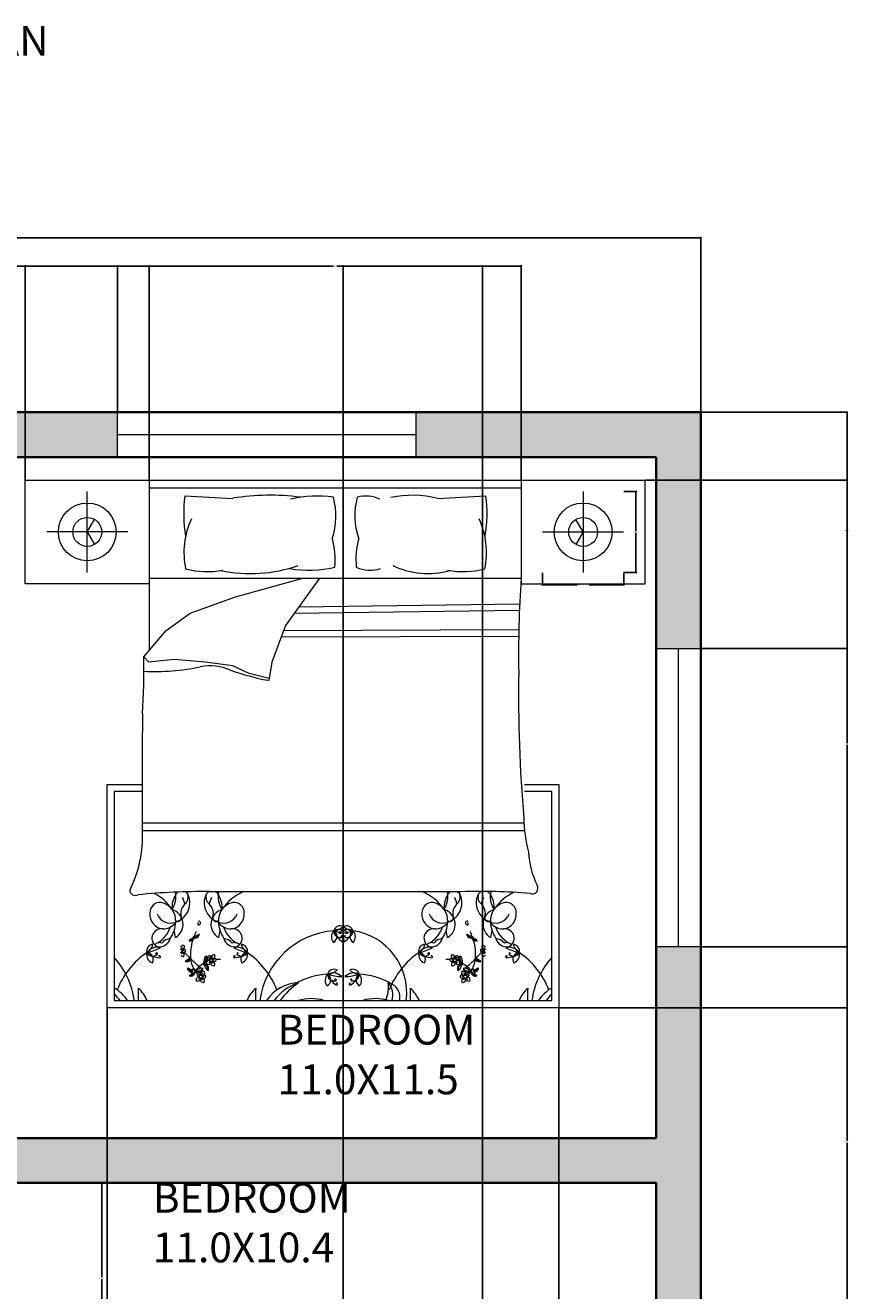
# Model space of a CAD drawing. Units: inches. Extents: x 0 to 423, y -517 to 94.
# Tile 8 of 8: x 257 to 423, y -160 to 94. Entities that reach past the tile are written whole.
import ezdxf

# ---------------------------------------------------------------- set-up
doc = ezdxf.new("R2010")
doc.units = ezdxf.units.IN
doc.header["$MEASUREMENT"] = 0
for name, color, linetype, lineweight in [('A-ANNO-DIMS', 2, 'Continuous', 18), ('A-ANNO-TEXT', 7, 'Continuous', 25), ('A-AREA-IDEN', 7, 'Continuous', 18), ('A-FURN', 8, 'Continuous', 13), ('A-GLAZ', 4, 'Continuous', 18), ('A-WALL', 7, 'Continuous', 35)]:
    doc.layers.add(name, color=color, linetype=linetype, lineweight=lineweight)
doc.layers.add('A-WALL-PATT', color=30, linetype='Continuous', lineweight=13, true_color=0xf26722)
doc.styles.get("Standard").update_dxf_attribs({"font": 'arial.ttf'})
doc.dimstyles.get("Standard").update_dxf_attribs({"dimtxt": 0.18, "dimasz": 0.18, "dimexe": 0.18, "dimexo": 0.0625, "dimgap": 0.09, "dimtad": 0, "dimtih": 1, "dimtoh": 1, "dimdec": 0, "dimzin": 0, "dimdsep": 46, "dimlunit": 3, "dimtxsty": 'Standard', "dimcen": 0.09, "dimadec": 0, "dimazin": 0, "dimtfac": 1, "dimtdec": 0, "dimtofl": 0, "dimtmove": 0, "dimatfit": 3, "dimfxl": 1, "dimtolj": 1, "dimtzin": 0, "dimarcsym": 0})

# ---------------------------------------------------------------- blocks, each defined once
blk = doc.blocks.new('*D1')
at = {"layer": 'A-ANNO-DIMS', "color": 0, "lineweight": -2, "transparency": 16777216}
for p, q in [((29.72, 16.3), (29.72, 51.54)), ((29.9, 51.36), (200.83, 51.36)), ((392.54, 51.36), (221.62, 51.36)), ((392.72, 16.3), (392.72, 51.54))]:
    blk.add_line(p, q, dxfattribs=at)
at = {"layer": 'A-ANNO-DIMS', "color": 0, "transparency": 16777216}
for points in [[(29.9, 51.39), (29.9, 51.33), (29.72, 51.36)], [(392.54, 51.39), (392.54, 51.33), (392.72, 51.36)]]:
    blk.add_solid(points, dxfattribs=at)
at = {"layer": 'Defpoints', "color": 0, "transparency": 16777216}
for p in [(392.72, 51.36), (29.72, 16.23), (392.72, 16.23)]:
    blk.add_point(p, dxfattribs=at)
at = {"layer": 'A-ANNO-DIMS', "color": 0, "transparency": 16777216, "insert": (211.22, 51.36), "char_height": 6, "attachment_point": 5}
blk.add_mtext('\\A1;30\'-3"', dxfattribs=at)
blk = doc.blocks.new('WIN-GLAZ-60IN')
for p, q in [((0, 60), (0, 0)), ((4.5, 60), (4.5, 0)), ((9, 0), (9, 60))]:
    blk.add_line(p, q)
blk = doc.blocks.new('BEDSIDE-LAMP-LARGE')
for p, q in [((8.15, 0), (8.15, 16.3)), ((16.3, 8.15), (0, 8.15))]:
    blk.add_line(p, q)
for points in [[(8.15, 8.15), (9.61, 10.67)], [(8.15, 8.15), (9.61, 5.63)]]:
    blk.add_lwpolyline(points)
for radius in [5.82, 2.91]:
    blk.add_circle((8.15, 8.15), radius)
blk = doc.blocks.new('*D28')
at = {"layer": 'A-ANNO-DIMS', "color": 0, "lineweight": -2, "transparency": 16777216}
for p, q in [((360.85, -16.06), (360.85, -18.62)), ((377.16, -16.06), (377.16, -18.62)), ((361.03, -18.44), (367.78, -18.44)), ((376.98, -18.44), (370.23, -18.44))]:
    blk.add_line(p, q, dxfattribs=at)
at = {"layer": 'A-ANNO-DIMS', "color": 0, "transparency": 16777216}
for points in [[(361.03, -18.41), (361.03, -18.47), (360.85, -18.44)], [(376.98, -18.41), (376.98, -18.47), (377.16, -18.44)]]:
    blk.add_solid(points, dxfattribs=at)
at = {"layer": 'Defpoints', "color": 0, "transparency": 16777216}
for p in [(360.85, -15.99), (377.16, -15.99), (360.85, -18.44)]:
    blk.add_point(p, dxfattribs=at)
at = {"layer": 'A-ANNO-DIMS', "color": 0, "transparency": 16777216, "insert": (369, -18.44), "char_height": 0.18, "attachment_point": 5}
blk.add_mtext('\\A1;LAMP 1\'-4 1/2" TYP.', dxfattribs=at)
blk = doc.blocks.new('*D29')
at = {"layer": 'A-ANNO-DIMS', "color": 0, "lineweight": -2, "transparency": 16777216}
for p, q in [((377.22, 0.31), (379.78, 0.31)), ((379.6, 0.13), (379.6, -7.66)), ((379.6, -15.81), (379.6, -8.03)), ((377.22, -15.99), (379.78, -15.99))]:
    blk.add_line(p, q, dxfattribs=at)
at = {"layer": 'A-ANNO-DIMS', "color": 0, "transparency": 16777216}
for points in [[(379.57, 0.13), (379.63, 0.13), (379.6, 0.31)], [(379.57, -15.81), (379.63, -15.81), (379.6, -15.99)]]:
    blk.add_solid(points, dxfattribs=at)
at = {"layer": 'Defpoints', "color": 0, "transparency": 16777216}
for p in [(377.16, 0.31), (377.16, -15.99), (379.6, -15.99)]:
    blk.add_point(p, dxfattribs=at)
at = {"layer": 'A-ANNO-DIMS', "color": 0, "transparency": 16777216, "insert": (379.6, -7.84), "char_height": 0.18, "attachment_point": 5}
blk.add_mtext('\\A1;1\'-4 1/2" TYP.', dxfattribs=at)
blk = doc.blocks.new('*D35')
at = {"layer": 'A-ANNO-DIMS', "color": 0, "lineweight": -2, "transparency": 16777216}
for p, q in [((320.72, -389.7), (320.72, 45.81)), ((320.9, 45.63), (334.39, 45.63)), ((348.54, 45.63), (335.05, 45.63)), ((348.72, -389.7), (348.72, 45.81))]:
    blk.add_line(p, q, dxfattribs=at)
at = {"layer": 'A-ANNO-DIMS', "color": 0, "transparency": 16777216}
for points in [[(320.9, 45.66), (320.9, 45.6), (320.72, 45.63)], [(348.54, 45.66), (348.54, 45.6), (348.72, 45.63)]]:
    blk.add_solid(points, dxfattribs=at)
at = {"layer": 'Defpoints', "color": 0, "transparency": 16777216}
for p in [(348.72, 45.63), (320.72, -389.77), (348.72, -389.77)]:
    blk.add_point(p, dxfattribs=at)
at = {"layer": 'A-ANNO-DIMS', "color": 0, "transparency": 16777216, "insert": (334.72, 45.63), "char_height": 0.18, "attachment_point": 5}
blk.add_mtext('\\A1;2\'-4"', dxfattribs=at)
blk = doc.blocks.new('*D40')
at = {"layer": 'A-ANNO-DIMS', "color": 0, "lineweight": -2, "transparency": 16777216}
for p, q in [((225.52, 16.3), (225.52, 45.81)), ((225.7, 45.63), (250.08, 45.63)), ((275.13, 45.63), (250.75, 45.63)), ((275.31, 16.3), (275.31, 45.81))]:
    blk.add_line(p, q, dxfattribs=at)
at = {"layer": 'A-ANNO-DIMS', "color": 0, "transparency": 16777216}
for points in [[(225.7, 45.66), (225.7, 45.6), (225.52, 45.63)], [(275.13, 45.66), (275.13, 45.6), (275.31, 45.63)]]:
    blk.add_solid(points, dxfattribs=at)
at = {"layer": 'Defpoints', "color": 0, "transparency": 16777216}
for p in [(275.31, 45.63), (225.52, 16.23), (275.31, 16.23)]:
    blk.add_point(p, dxfattribs=at)
at = {"layer": 'A-ANNO-DIMS', "color": 0, "transparency": 16777216, "insert": (250.41, 45.63), "char_height": 0.18, "attachment_point": 5}
blk.add_mtext('\\A1;4\'-2"', dxfattribs=at)
blk = doc.blocks.new('*D42')
at = {"layer": 'A-ANNO-DIMS', "color": 0, "lineweight": -2, "transparency": 16777216}
for p, q in [((392.79, 16.23), (422.3, 16.23)), ((422.12, 16.05), (422.12, -7.33)), ((422.12, -31.09), (422.12, -7.7)), ((392.79, -31.27), (422.3, -31.27))]:
    blk.add_line(p, q, dxfattribs=at)
at = {"layer": 'A-ANNO-DIMS', "color": 0, "transparency": 16777216}
for points in [[(422.09, 16.05), (422.15, 16.05), (422.12, 16.23)], [(422.09, -31.09), (422.15, -31.09), (422.12, -31.27)]]:
    blk.add_solid(points, dxfattribs=at)
at = {"layer": 'Defpoints', "color": 0, "transparency": 16777216}
for p in [(392.72, 16.23), (392.72, -31.27), (422.12, -31.27)]:
    blk.add_point(p, dxfattribs=at)
at = {"layer": 'A-ANNO-DIMS', "color": 0, "transparency": 16777216, "insert": (422.12, -7.52), "char_height": 0.18, "attachment_point": 5}
blk.add_mtext('\\A1;3\'-11 1/2"', dxfattribs=at)
blk = doc.blocks.new('*D43')
at = {"layer": 'A-ANNO-DIMS', "color": 0, "lineweight": -2, "transparency": 16777216}
for p, q in [((392.79, -91.27), (422.3, -91.27)), ((422.12, -91.45), (422.12, -130.33)), ((422.12, -169.59), (422.12, -130.7)), ((392.79, -169.77), (422.3, -169.77))]:
    blk.add_line(p, q, dxfattribs=at)
at = {"layer": 'A-ANNO-DIMS', "color": 0, "transparency": 16777216}
for points in [[(422.09, -91.45), (422.15, -91.45), (422.12, -91.27)], [(422.09, -169.59), (422.15, -169.59), (422.12, -169.77)]]:
    blk.add_solid(points, dxfattribs=at)
at = {"layer": 'Defpoints', "color": 0, "transparency": 16777216}
for p in [(392.72, -91.27), (392.72, -169.77), (422.12, -169.77)]:
    blk.add_point(p, dxfattribs=at)
at = {"layer": 'A-ANNO-DIMS', "color": 0, "transparency": 16777216, "insert": (422.12, -130.52), "char_height": 0.18, "attachment_point": 5}
blk.add_mtext('\\A1;6\'-6 1/2"', dxfattribs=at)
blk = doc.blocks.new('*D50')
at = {"layer": 'A-ANNO-DIMS', "color": 0, "lineweight": -2, "transparency": 16777216}
for p, q in [((273.19, -103.61), (273.19, -517.35)), ((364.14, -103.61), (364.14, -517.35)), ((273.37, -517.17), (318.34, -517.17)), ((363.96, -517.17), (318.99, -517.17))]:
    blk.add_line(p, q, dxfattribs=at)
at = {"layer": 'A-ANNO-DIMS', "color": 0, "transparency": 16777216}
for points in [[(273.37, -517.14), (273.37, -517.2), (273.19, -517.17)], [(363.96, -517.14), (363.96, -517.2), (364.14, -517.17)]]:
    blk.add_solid(points, dxfattribs=at)
at = {"layer": 'Defpoints', "color": 0, "transparency": 16777216}
for p in [(273.19, -103.55), (364.14, -103.55), (364.14, -517.17)]:
    blk.add_point(p, dxfattribs=at)
at = {"layer": 'A-ANNO-DIMS', "color": 0, "transparency": 16777216, "insert": (318.66, -517.17), "char_height": 0.18, "attachment_point": 5}
blk.add_mtext('\\A1;7\'-7"', dxfattribs=at)
blk = doc.blocks.new('*D55')
at = {"layer": 'A-ANNO-DIMS', "color": 0, "lineweight": -2, "transparency": 16777216}
for p, q in [((242.79, -138.77), (272.3, -138.77)), ((272.12, -138.95), (272.12, -157.77)), ((272.12, -176.96), (272.12, -158.14)), ((242.79, -177.14), (272.3, -177.14))]:
    blk.add_line(p, q, dxfattribs=at)
at = {"layer": 'A-ANNO-DIMS', "color": 0, "transparency": 16777216}
for points in [[(272.09, -138.95), (272.15, -138.95), (272.12, -138.77)], [(272.09, -176.96), (272.15, -176.96), (272.12, -177.14)]]:
    blk.add_solid(points, dxfattribs=at)
at = {"layer": 'Defpoints', "color": 0, "transparency": 16777216}
for p in [(242.72, -138.77), (242.72, -177.14), (272.12, -177.14)]:
    blk.add_point(p, dxfattribs=at)
at = {"layer": 'A-ANNO-DIMS', "color": 0, "transparency": 16777216, "insert": (272.12, -157.95), "char_height": 0.18, "attachment_point": 5}
blk.add_mtext('\\A1;3\'-2 1/2"', dxfattribs=at)
blk = doc.blocks.new('*D60')
at = {"layer": 'A-ANNO-DIMS', "color": 0, "lineweight": -2, "transparency": 16777216}
for p, q in [((381.54, 2.55), (422.3, 2.55)), ((422.12, 2.37), (422.12, -50.32)), ((422.12, -103.37), (422.12, -50.68)), ((364.2, -103.55), (422.3, -103.55))]:
    blk.add_line(p, q, dxfattribs=at)
at = {"layer": 'A-ANNO-DIMS', "color": 0, "transparency": 16777216}
for points in [[(422.09, 2.37), (422.15, 2.37), (422.12, 2.55)], [(422.09, -103.37), (422.15, -103.37), (422.12, -103.55)]]:
    blk.add_solid(points, dxfattribs=at)
at = {"layer": 'Defpoints', "color": 0, "transparency": 16777216}
for p in [(381.48, 2.55), (364.14, -103.55), (422.12, -103.55)]:
    blk.add_point(p, dxfattribs=at)
at = {"layer": 'A-ANNO-DIMS', "color": 0, "transparency": 16777216, "insert": (422.12, -50.5), "char_height": 0.18, "attachment_point": 5}
blk.add_mtext('\\A1;8\'-10"', dxfattribs=at)
blk = doc.blocks.new('*D62')
at = {"layer": 'A-ANNO-DIMS', "color": 0, "lineweight": -2, "transparency": 16777216}
for p, q in [((256.72, 2.62), (256.72, 45.81)), ((256.9, 45.63), (268.86, 45.63)), ((281.49, 45.63), (269.53, 45.63)), ((281.67, 2.62), (281.67, 45.81))]:
    blk.add_line(p, q, dxfattribs=at)
at = {"layer": 'A-ANNO-DIMS', "color": 0, "transparency": 16777216}
for points in [[(256.9, 45.66), (256.9, 45.6), (256.72, 45.63)], [(281.49, 45.66), (281.49, 45.6), (281.67, 45.63)]]:
    blk.add_solid(points, dxfattribs=at)
at = {"layer": 'Defpoints', "color": 0, "transparency": 16777216}
for p in [(281.67, 45.63), (256.72, 2.55), (281.67, 2.55)]:
    blk.add_point(p, dxfattribs=at)
at = {"layer": 'A-ANNO-DIMS', "color": 0, "transparency": 16777216, "insert": (269.19, 45.63), "char_height": 0.18, "attachment_point": 5}
blk.add_mtext('\\A1;2\'-1"', dxfattribs=at)
blk = doc.blocks.new('*D64')
at = {"layer": 'A-ANNO-DIMS', "color": 0, "lineweight": -2, "transparency": 16777216}
for p, q in [((281.67, 2.62), (281.67, 45.81)), ((281.85, 45.63), (318.77, 45.63)), ((356.35, 45.63), (319.43, 45.63)), ((356.53, 2.62), (356.53, 45.81))]:
    blk.add_line(p, q, dxfattribs=at)
at = {"layer": 'A-ANNO-DIMS', "color": 0, "transparency": 16777216}
for points in [[(281.85, 45.66), (281.85, 45.6), (281.67, 45.63)], [(356.35, 45.66), (356.35, 45.6), (356.53, 45.63)]]:
    blk.add_solid(points, dxfattribs=at)
at = {"layer": 'Defpoints', "color": 0, "transparency": 16777216}
for p in [(356.53, 45.63), (281.67, 2.55), (356.53, 2.55)]:
    blk.add_point(p, dxfattribs=at)
at = {"layer": 'A-ANNO-DIMS', "color": 0, "transparency": 16777216, "insert": (319.1, 45.63), "char_height": 0.18, "attachment_point": 5}
blk.add_mtext('\\A1;6\'-3"', dxfattribs=at)

msp = doc.modelspace()

# ---------------------------------------------------------------- hatches: boundary and pattern name
at = {"layer": 'A-WALL-PATT'}
h = msp.add_hatch(color=256, dxfattribs=at)
h.dxf.hatch_style = 1
h.paths.add_polyline_path([(201.52, 16.23), (138.22, 16.23), (138.22, 7.23), (177.72, 7.23), (177.72, -138.77), (186.72, -138.77), (186.72, -92.77), (251.72, -92.77), (251.72, -22.53), (242.72, -22.53), (242.72, -83.77), (186.72, -83.77), (186.72, 7.23), (201.52, 7.23)])
h.paths.add_polyline_path([(78.22, 16.23), (29.72, 16.23), (29.72, -31.27), (38.72, -31.27), (38.72, 7.23), (78.22, 7.23)])
h.paths.add_polyline_path([(275.31, 16.23), (225.52, 16.23), (225.52, 7.23), (275.31, 7.23)])
h.paths.add_polyline_path([(392.72, 16.23), (335.31, 16.23), (335.31, 7.23), (383.72, 7.23), (383.72, -31.27), (392.72, -31.27)])
h.paths.add_polyline_path([(143.33, -129.77), (38.72, -129.77), (38.72, -91.27), (29.72, -91.27), (29.72, -157.27), (38.72, -157.27), (38.72, -138.77), (143.33, -138.77)])
h.paths.add_polyline_path([(186.72, -199.77), (38.72, -199.77), (38.72, -181.27), (29.72, -181.27), (29.72, -239.27), (38.72, -239.27), (38.72, -208.77), (177.72, -208.77), (177.72, -237.07), (186.72, -237.07)])
h.paths.add_polyline_path([(111.72, -161.55), (102.72, -161.55), (102.72, -199.77), (111.72, -199.77)])
h.paths.add_polyline_path([(392.72, -91.27), (383.72, -91.27), (383.72, -129.77), (242.72, -129.77), (242.72, -138.77), (383.72, -138.77), (383.72, -169.77), (392.72, -169.77)])
h.paths.add_polyline_path([(392.72, -229.77), (383.72, -229.77), (383.72, -262.77), (251.72, -262.77), (251.72, -177.14), (242.72, -177.14), (242.72, -271.77), (383.72, -271.77), (383.72, -300.77), (392.72, -300.77)])
h.paths.add_polyline_path([(392.72, -360.77), (383.72, -360.77), (383.72, -389.77), (378.42, -389.77), (378.42, -398.77), (383.72, -398.77), (383.72, -458.77), (382.72, -458.77), (382.72, -467.77), (392.72, -467.77)])
h.paths.add_polyline_path([(364.92, -389.77), (348.72, -389.77), (348.72, -467.77), (358.72, -467.77), (358.72, -458.77), (357.72, -458.77), (357.72, -398.77), (364.92, -398.77)])
h.paths.add_polyline_path([(320.72, -389.77), (283.72, -389.77), (283.72, -398.77), (320.72, -398.77)])
h.paths.add_polyline_path([(223.72, -389.77), (186.72, -389.77), (186.72, -270.38), (177.72, -270.38), (177.72, -458.77), (138.22, -458.77), (138.22, -467.77), (186.72, -467.77), (186.72, -398.77), (223.72, -398.77)])
h.paths.add_polyline_path([(143.29, -329.77), (38.72, -329.77), (38.72, -299.27), (29.72, -299.27), (29.72, -338.77), (143.29, -338.77)])
h.paths.add_polyline_path([(38.72, -374.71), (29.72, -374.71), (29.72, -398.74), (38.72, -398.74)])
h.paths.add_polyline_path([(78.22, -458.77), (38.72, -458.77), (38.72, -434.74), (29.72, -434.74), (29.72, -467.77), (78.22, -467.77)])
h.paths.add_polyline_path([(279.99, -158.17), (326.6, -158.17), (326.6, -135.78), (279.99, -135.78)], flags=25)
h.paths.add_polyline_path([(355.56, -439.13), (387, -439.13), (387, -416.66), (355.56, -416.66)], flags=9)

# ---------------------------------------------------------------- linework, layer by layer
at = {"layer": 'A-FURN'}
for p, q in [((256.72, 2.55), (381.48, 2.55)), ((281.67, 2.55), (281.67, -31.69)), ((356.53, 0.95), (281.67, 0.95)), ((281.67, -17.16), (356.53, -17.16)), ((299, -20.87), (312.61, -17.16)), ((315.95, -17.16), (309.11, -26.68)), ((289.9, -24.15), (299, -20.87)), ((356.19, -22.35), (311.77, -22.97)), ((285.1, -27.69), (289.9, -24.15)), ((356.14, -23.63), (310.84, -24.27)), ((280.55, -32.99), (285.1, -27.69)), ((309.11, -26.68), (306.33, -34)), ((356.08, -27.55), (308.71, -27.74)), ((356.09, -28.84), (308.22, -29.03)), ((281.56, -34), (280.55, -32.99)), ((286.62, -33.5), (281.56, -34)), ((292.94, -34), (286.62, -33.5)), ((298.5, -34.76), (292.94, -34)), ((301.78, -36.28), (298.5, -34.76)), ((306.33, -34), (305.82, -37.29)), ((305.82, -37.29), (301.78, -36.28)), ((273.19, -58.61), (280.24, -58.61)), ((273.19, -103.55), (273.19, -58.61)), ((280.24, -60.05), (274.63, -60.05)), ((274.63, -60.05), (274.63, -102.1)), ((362.7, -60.05), (357.2, -60.05)), ((357.22, -58.61), (364.14, -58.61)), ((362.7, -102.1), (362.7, -60.05)), ((364.14, -58.61), (364.14, -103.55)), ((357.09, -66.39), (280.23, -66.39)), ((357.21, -67.94), (280.23, -67.94)), ((344.43, -80.2), (293.77, -80.2)), ((286.93, -89.45), (286.65, -88.04)), ((295.65, -89.45), (295.92, -88.04)), ((341.68, -89.45), (341.41, -88.04)), ((350.4, -89.45), (350.68, -88.04)), ((364.14, -103.55), (273.19, -103.55)), ((274.63, -102.1), (362.7, -102.1))]:
    msp.add_line(p, q, dxfattribs=at)
for points in [[(281.67, -18.24), (256.72, -18.24), (256.72, 2.55)], [(356.53, 2.55), (356.53, -18.24), (381.48, -18.24), (381.48, 2.55)]]:
    msp.add_lwpolyline(points, dxfattribs=at)
for points in [[(288.84, -0.56, 0.074897), (288.99, -8.71, -0.472817)], [(318.51, -9.16, 0.14099), (318.76, -0.85, 0.235245)], [(323.84, -9.16, -0.14099), (323.59, -0.85, -0.235245)], [(349.36, -0.56, -0.074897), (349.21, -8.71, 0.472817)], [(280.29, -44.42, 0.001242), (280.23, -68.09, -0.127202), (277.73, -79.89)], [(357.06, -65.4, 0.056112), (357.97, -72.27, 0.095341), (359.72, -78.88)]]:
    msp.add_lwpolyline(points, format="xyb", dxfattribs=at)
for centre in [(294.13, -93.97), (343.19, -93.97), (292.06, -97.32), (345.27, -97.32)]:
    msp.add_circle(centre, 0.318, dxfattribs=at)
for centre, radius, start, end in [((357.6, 1186.76), 1189.31, 266.68521, 267.14978), ((305.93, -45.7), 45.25, 82.2196, 99.497), ((315.49, -22.84), 22.23, 81.5249, 103.96), ((325.3, -6.78), 6.17, 63.3437, 106.1026), ((334.55, -22.39), 21.93, 76.3427, 101.1841), ((280.59, 1186.76), 1189.31, 272.85022, 273.31479), ((304.73, -11.98), 16.08, 155.1316, 191.7583), ((333.47, -11.98), 16.08, 348.2417, 24.8684), ((303.81, -13.33), 15.29, 354.0129, 15.8293), ((338.55, -13.33), 15.29, 164.1707, 185.9871), ((293.29, 0.9), 16.72, 255.1039, 281.0369), ((302.09, 12.79), 29, 258.0397, 289.2615), ((313.83, 6.46), 22, 259.8617, 283.6238), ((326.14, -8.93), 6.61, 245.0183, 288.5407), ((337.7, -0.33), 15.88, 243.8761, 286.1746), ((344.91, 0.9), 16.72, 258.9631, 284.8961), ((580.18, -32.41), 224.18, 176.1, 180.9282), ((166.16, -36.09), 114.44, 355.8294, 1.553), ((282.69, 11.19), 47.09, 267.4519, 281.3392), ((293.94, -44.94), 10.16, 66.2616, 101.3392), ((314.49, 9.86), 48.38, 250.1194, 259.3383), ((305.54, -37.39), 0.301, 268.8623, 19.7536), ((648.43, -40.56), 292.43, 179.1145, 184.8735), ((358.77, -79.51), 1.14, 246.5219, 33.8264), ((278.88, -79.81), 1.15, 183.98, 297.3412), ((292.28, -210.07), 129.88, 89.3433, 95.6887), ((278.39, -88.98), 9.44, 33.6671, 63.2997), ((291.05, -83.36), 4.81, 145.785, 184.7304), ((281.86, -81.12), 5.17, 328.8218, 9.1554), ((288.26, -81.58), 1.5, 120.0293, 142.325), ((285.86, -82.46), 3.98, 289.2822, 29.1751), ((285.26, -83.18), 3.59, 7.436, 29.9149), ((287.62, -81.28), 1.87, 311.5653, 23.8354), ((288.26, -81.58), 1.5, 44.4517, 63.558), ((296.71, -82.46), 3.98, 150.8249, 250.7178), ((294.95, -81.28), 1.87, 156.1646, 228.4347), ((294.31, -81.58), 1.5, 113.229, 135.5483), ((297.31, -83.18), 3.59, 150.0851, 172.564), ((294.31, -81.58), 1.5, 37.675, 66.7144), ((291.52, -83.36), 4.81, 355.2696, 34.215), ((300.71, -81.12), 5.17, 169.7133, 211.1782), ((304.18, -88.98), 9.44, 111.4941, 146.3329), ((333.15, -88.98), 9.44, 33.6671, 68.5059), ((345.81, -83.36), 4.81, 145.785, 184.7304), ((336.61, -81.12), 5.17, 328.8218, 10.2867), ((343.02, -81.58), 1.5, 113.2856, 142.325), ((340.62, -82.46), 3.98, 289.2822, 29.1751), ((340.02, -83.18), 3.59, 7.436, 29.9149), ((343.02, -81.58), 1.5, 44.4517, 66.7144), ((342.38, -81.28), 1.87, 311.5653, 23.8354), ((348.25, -201.54), 121.4, 85.2402, 91.8035), ((351.47, -82.46), 3.98, 150.8249, 250.7178), ((349.7, -81.28), 1.87, 156.1646, 228.4347), ((349.07, -81.58), 1.5, 106.6343, 135.5483), ((352.07, -83.18), 3.59, 150.0851, 172.564), ((349.07, -81.58), 1.5, 37.675, 72.5814), ((346.28, -83.36), 4.81, 355.2696, 34.215), ((355.47, -81.12), 5.17, 169.249, 211.1782), ((358.93, -88.98), 9.44, 113.6453, 146.3329), ((283.89, -84.45), 2.11, 84.4856, 181.0538), ((283.25, -86.01), 3.75, 355.2933, 76.921), ((285.38, -86.76), 3.1, 299.9085, 73.1337), ((290.56, -84.59), 2.56, 131.5653, 195.1471), ((292.01, -84.59), 2.56, 344.8529, 48.4347), ((297.19, -86.76), 3.1, 106.8663, 240.0915), ((299.32, -86.01), 3.75, 103.079, 184.7067), ((298.68, -84.45), 2.11, 358.9462, 95.5144), ((338.65, -84.45), 2.11, 84.4856, 181.0538), ((338, -86.01), 3.75, 355.2933, 76.921), ((340.14, -86.76), 3.1, 299.9085, 73.1337), ((345.32, -84.59), 2.56, 131.5653, 195.1471), ((346.77, -84.59), 2.56, 344.8529, 48.4347), ((351.95, -86.76), 3.1, 106.8663, 240.0915), ((354.08, -86.01), 3.75, 103.079, 184.7067), ((353.43, -84.45), 2.11, 358.9462, 95.5144), ((284.76, -84.75), 2.98, 174.9449, 262.8857), ((285.93, -83.62), 2.9, 201.5819, 291.4221), ((284.24, -84.09), 3.62, 272.3591, 324.0401), ((280.31, -85.91), 6.7, 326.2883, 356.5076), ((291.05, -83.36), 4.81, 212.7011, 216.3445), ((287.34, -85.46), 0.774, 257.3041, 15.1471), ((291.64, -86.64), 0.24, 102.7051, 280.4384), ((291.62, -86.49), 0.391, 280.4384, 100.4136), ((295.23, -85.46), 0.774, 164.8529, 282.6959), ((291.52, -83.36), 4.81, 323.6555, 327.2989), ((298.33, -84.09), 3.62, 215.9599, 267.6409), ((296.64, -83.62), 2.9, 248.5779, 338.4181), ((302.27, -85.91), 6.7, 183.4924, 213.7117), ((297.81, -84.75), 2.98, 277.1143, 5.0551), ((339.51, -84.75), 2.98, 174.9449, 262.8857), ((340.69, -83.62), 2.9, 201.5819, 291.4221), ((339, -84.09), 3.62, 272.3591, 324.0401), ((335.06, -85.91), 6.7, 326.2883, 356.5076), ((345.81, -83.36), 4.81, 212.7011, 216.3445), ((342.1, -85.46), 0.774, 257.3041, 15.1471), ((345.71, -86.49), 0.391, 79.5864, 259.5616), ((345.68, -86.64), 0.24, 259.5616, 77.2949), ((349.98, -85.46), 0.774, 164.8529, 282.6959), ((346.28, -83.36), 4.81, 323.6555, 327.2989), ((353.09, -84.09), 3.62, 215.9599, 267.6409), ((351.4, -83.62), 2.9, 248.5779, 338.4181), ((357.02, -85.91), 6.7, 183.4924, 213.7117), ((352.57, -84.75), 2.98, 277.1143, 5.0551), ((284.07, -89.55), 1.87, 80.264, 250.8688), ((280.36, -85.43), 5.89, 301.2614, 341.7045), ((300.29, -92.92), 10.33, 153.0032, 159.8941), ((290.47, -87.2), 2, 285.5129, 293.6099), ((291.77, -89.45), 0.655, 87.3579, 140.4944), ((290.26, -87.57), 1.97, 301.164, 321.5612), ((288.66, -87.22), 3.52, 324.6898, 333.4936), ((302.21, -85.43), 5.89, 198.2955, 238.7386), ((298.5, -89.55), 1.87, 289.1312, 99.736), ((320.07, -104.3), 16.29, 94.4623, 172.255), ((320.14, -89.27), 1.81, 137.7873, 219.1145), ((318.09, -89.21), 1.36, 298.5391, 58.3627), ((320.1, -88.43), 1.35, 63.0274, 163.8037), ((318.73, -85.27), 2.78, 271.4585, 315.3727), ((319.86, -90.4), 2.58, 45.5411, 114.3101), ((322.21, -77.18), 11.4, 252.593, 267.2582), ((320.13, -88.11), 1.33, 177.7585, 283.852), ((322.7, -86.72), 4.12, 198.9159, 238.011), ((321.62, -90.4), 2.58, 65.6899, 134.4589), ((319.28, -77.18), 11.4, 272.7418, 287.407), ((320.41, -89.23), 0.176, 283.852, 219.9245), ((321.39, -88.43), 1.35, 16.1963, 116.9726), ((322.76, -85.27), 2.78, 224.6273, 268.5415), ((321.06, -89.16), 0.106, 320.1909, 256.0209), ((318.79, -86.72), 4.12, 301.989, 341.0841), ((321.35, -88.11), 1.33, 256.148, 2.2415), ((323.4, -89.21), 1.36, 121.6373, 241.4609), ((321.35, -89.27), 1.81, 320.8855, 42.2127), ((320.89, -100.54), 12.61, 352.8636, 81.8197), ((338.83, -89.55), 1.87, 80.264, 250.8688), ((335.12, -85.43), 5.89, 301.2614, 341.7045), ((347.07, -87.57), 1.97, 218.4388, 238.836), ((345.55, -89.45), 0.655, 39.5056, 92.6421), ((348.67, -87.22), 3.52, 206.5064, 215.3102), ((346.86, -87.2), 2, 246.3901, 254.4871), ((337.04, -92.92), 10.33, 20.1059, 26.9968), ((356.97, -85.43), 5.89, 198.2955, 238.7386), ((353.26, -89.55), 1.87, 289.1312, 99.736), ((282.49, -92.14), 1.35, 92.9516, 193.728), ((279.73, -90.09), 2.78, 301.3827, 345.2969), ((283.26, -93.97), 2.58, 75.4653, 144.2343), ((278.7, -81.34), 11.4, 282.5173, 297.1824), ((283.69, -91.58), 1.15, 63.9755, 143.2681), ((283.62, -88.99), 2.34, 265.969, 344.3045), ((286.14, -92.1), 2.49, 96.1662, 141.5825), ((288.41, -91.59), 0.53, 101.5637, 142.6358), ((288.34, -91.79), 0.303, 91.1081, 181.8675), ((287.99, -91.18), 0.764, 288.7263, 352.5032), ((288.51, -91.22), 0.245, 345.2356, 144.9248), ((290.27, -90.35), 0.655, 101.3256, 154.4621), ((289.32, -88.13), 1.97, 280.2588, 300.656), ((289.78, -86.55), 3.52, 268.3264, 277.1302), ((300.29, -92.92), 10.33, 163.5842, 183.8277), ((288.9, -88.14), 2, 308.2101, 316.3071), ((290.13, -89.45), 0.599, 278.3432, 4.2869), ((289.8, -88.93), 1.05, 300.656, 332.6341), ((290.58, -89.62), 0.254, 55.7657, 157.4417), ((290.98, -89.38), 0.254, 84.3784, 186.0543), ((290.74, -88.36), 1.05, 269.1859, 301.164), ((291.05, -88.9), 0.599, 237.5332, 323.4768), ((296.43, -92.1), 2.49, 38.4175, 83.8338), ((298.95, -88.99), 2.34, 195.6955, 274.031), ((298.88, -91.58), 1.15, 36.7319, 116.0245), ((299.31, -93.97), 2.58, 35.7657, 104.5347), ((303.87, -81.34), 11.4, 242.8176, 257.4827), ((300.09, -92.14), 1.35, 346.272, 87.0484), ((302.85, -90.09), 2.78, 194.7031, 238.6173), ((320.62, -90.04), 0.202, 238.011, 71.5592), ((320.66, -89.94), 0.0983, 71.5592, 188.0167), ((320.86, -90.04), 0.202, 108.4408, 301.989), ((320.83, -89.94), 0.0983, 351.9833, 108.4408), ((337.24, -92.14), 1.35, 92.9516, 193.728), ((334.48, -90.09), 2.78, 301.3827, 345.2969), ((338.02, -93.97), 2.58, 75.4653, 144.2343), ((333.46, -81.34), 11.4, 282.5173, 297.1824), ((338.44, -91.58), 1.15, 63.9755, 143.2681), ((338.38, -88.99), 2.34, 265.969, 344.3045), ((340.9, -92.1), 2.49, 96.1662, 141.5825), ((346.28, -88.9), 0.599, 216.5232, 302.4668), ((346.59, -88.36), 1.05, 238.836, 270.8141), ((346.35, -89.38), 0.254, 353.9457, 95.6216), ((346.75, -89.62), 0.254, 22.5583, 124.2343), ((347.2, -89.45), 0.599, 175.7131, 261.6568), ((347.53, -88.93), 1.05, 207.3659, 239.344), ((337.04, -92.92), 10.33, 356.1723, 16.4158), ((348.43, -88.14), 2, 223.6929, 231.7899), ((348, -88.13), 1.97, 239.344, 259.7412), ((347.55, -86.55), 3.52, 262.8698, 271.6736), ((347.06, -90.35), 0.655, 25.5379, 78.6744), ((348.82, -91.22), 0.245, 35.0752, 194.7644), ((349.34, -91.18), 0.764, 187.4968, 251.2737), ((348.98, -91.79), 0.303, 358.1325, 88.8919), ((348.91, -91.59), 0.53, 37.3642, 78.4363), ((353.7, -88.99), 2.34, 195.6955, 274.031), ((351.19, -92.1), 2.49, 38.4175, 83.8338), ((353.64, -91.58), 1.15, 36.7319, 116.0245), ((354.06, -93.97), 2.58, 35.7657, 104.5347), ((358.62, -81.34), 11.4, 242.8176, 257.4827), ((357.6, -90.09), 2.78, 194.7031, 238.6173), ((354.84, -92.14), 1.35, 346.272, 87.0484), ((262.5, -104.3), 16.29, 7.745, 41.8856), ((290.38, -105.91), 16.29, 124.3865, 158.5908), ((282.94, -92.85), 1.81, 167.7115, 249.0387), ((281.13, -93.82), 1.36, 328.4633, 88.2869), ((283.89, -89.36), 4.12, 228.8402, 267.9352), ((282.35, -91.84), 1.33, 207.6827, 313.7762), ((283.15, -92.68), 0.176, 313.7762, 249.7183), ((283.72, -93.17), 0.0983, 101.4834, 217.9409), ((283.75, -93.28), 0.202, 267.9352, 101.4834), ((287.97, -92.09), 0.318, 273.2768, 86.7232), ((288.41, -92.67), 0.525, 217.7621, 259.0403), ((288.97, -91.98), 0.965, 203.4276, 227.6104), ((288.67, -92.4), 0.657, 80.3487, 133.6538), ((288.55, -91.85), 0.52, 229.7889, 317.6792), ((287.96, -92.95), 0.738, 355.053, 68.3618), ((288.54, -93.08), 1.04, 83.0852, 105.7171), ((288.46, -93), 0.244, 232.4737, 355.053), ((281.34, -101.71), 11.85, 43.1541, 52.0459), ((288.73, -92.02), 0.274, 317.6792, 80.3487), ((289.52, -94.55), 0.655, 101.3256, 154.4621), ((288.58, -92.33), 1.97, 280.2588, 300.656), ((288.15, -92.33), 2, 308.2101, 316.3071), ((289.38, -93.65), 0.599, 278.3432, 4.2869), ((289.05, -93.12), 1.05, 300.656, 332.6341), ((289.84, -93.82), 0.254, 55.7657, 157.4417), ((295.14, -93.18), 5.18, 184.756, 209.2041), ((302.6, -82.15), 17.05, 222.2412, 232.1744), ((291.7, -93.5), 1.45, 304.5369, 16.3699), ((292.48, -93.83), 0.88, 272.8499, 356.1226), ((291.85, -94.17), 0.852, 321.7607, 7.9252), ((293.71, -93.91), 1.02, 127.3105, 187.9252), ((292.31, -93.79), 1.05, 355.0106, 41.658), ((294.05, -94.93), 1, 104.7558, 148.0499), ((293.78, -93.53), 0.433, 126.1046, 271.4281), ((293.74, -93.41), 0.311, 353.7526, 131.7054), ((293.44, -93.78), 0.437, 0.0645, 61.1507), ((293.55, -93.41), 0.5, 311.8413, 355.7877), ((294.57, -93.48), 0.53, 101.5637, 176.365), ((294.5, -93.67), 0.303, 91.1081, 181.8675), ((294.83, -94.28), 0.657, 80.3487, 133.6538), ((294.71, -93.74), 0.52, 229.7889, 317.6792), ((294.15, -93.07), 0.764, 288.7263, 352.5032), ((294.12, -94.84), 0.738, 355.053, 68.3618), ((294.7, -94.97), 1.04, 83.0852, 105.7171), ((294.67, -93.1), 0.245, 345.2356, 144.9248), ((294.89, -93.91), 0.274, 317.6792, 80.3487), ((295.68, -100.06), 6.21, 87.1071, 94.7585), ((298.83, -93.28), 0.202, 78.5166, 272.0648), ((298.69, -89.36), 4.12, 272.0648, 311.1598), ((298.85, -93.17), 0.0983, 322.0591, 78.5166), ((300.22, -91.84), 1.33, 226.2238, 332.3173), ((299.44, -92.61), 0.106, 290.2667, 226.2271), ((301.44, -93.82), 1.36, 91.7131, 211.5367), ((299.63, -92.85), 1.81, 290.9613, 12.2885), ((292.2, -105.91), 16.29, 21.4092, 55.6135), ((345.13, -105.91), 16.29, 124.3865, 158.5908), ((337.7, -92.85), 1.81, 167.7115, 249.0387), ((337.11, -91.84), 1.33, 207.6827, 313.7762), ((338.64, -89.36), 4.12, 228.8402, 267.9352), ((335.89, -93.82), 1.36, 328.4633, 88.2869), ((337.91, -92.68), 0.176, 313.7762, 249.7183), ((338.48, -93.17), 0.0983, 101.4834, 217.9409), ((338.5, -93.28), 0.202, 267.9352, 101.4834), ((341.65, -100.06), 6.21, 85.2415, 92.8929), ((342.44, -93.91), 0.274, 99.6513, 222.3208), ((342.62, -93.74), 0.52, 222.3208, 310.2111), ((342.5, -94.28), 0.657, 46.3462, 99.6513), ((342.66, -93.1), 0.245, 35.0752, 194.7644), ((343.18, -93.07), 0.764, 187.4968, 251.2737), ((343.21, -94.84), 0.738, 111.6382, 184.947), ((342.63, -94.97), 1.04, 74.2829, 96.9148), ((342.82, -93.67), 0.303, 358.1325, 88.8919), ((342.75, -93.48), 0.53, 3.635, 78.4363), ((343.59, -93.41), 0.311, 48.2946, 186.2474), ((343.78, -93.41), 0.5, 184.2123, 228.1587), ((343.89, -93.78), 0.437, 118.8493, 179.9355), ((343.54, -93.53), 0.433, 268.5719, 53.8954), ((343.28, -94.93), 1, 31.9501, 75.2442), ((345.02, -93.79), 1.05, 138.342, 184.9894), ((344.85, -93.83), 0.88, 183.8774, 267.1501), ((345.63, -93.5), 1.45, 163.6301, 235.4631), ((343.62, -93.91), 1.02, 352.0748, 52.6895), ((345.47, -94.17), 0.852, 172.0748, 218.2393), ((334.73, -82.15), 17.05, 307.8256, 317.7588), ((342.18, -93.18), 5.18, 330.7959, 355.244), ((347.94, -93.65), 0.599, 175.7131, 261.6568), ((355.99, -101.71), 11.85, 127.9541, 136.8459), ((347.49, -93.82), 0.254, 22.5583, 124.2343), ((348.28, -93.12), 1.05, 207.3659, 239.344), ((349.17, -92.33), 2, 223.6929, 231.7899), ((348.75, -92.33), 1.97, 239.344, 259.7412), ((347.81, -94.55), 0.655, 25.5379, 78.6744), ((348.6, -92.02), 0.274, 99.6513, 222.3208), ((348.78, -91.85), 0.52, 222.3208, 310.2111), ((348.66, -92.4), 0.657, 46.3462, 99.6513), ((349.36, -92.95), 0.738, 111.6382, 184.947), ((348.87, -93), 0.244, 184.947, 307.5263), ((348.79, -93.08), 1.04, 74.2829, 96.9148), ((348.35, -91.98), 0.965, 312.3896, 336.5724), ((348.92, -92.67), 0.525, 280.9597, 322.2379), ((349.35, -92.09), 0.318, 93.2768, 266.7232), ((353.58, -93.28), 0.202, 78.5166, 272.0648), ((353.44, -89.36), 4.12, 272.0648, 311.1598), ((353.6, -93.17), 0.0983, 322.0591, 78.5166), ((354.97, -91.84), 1.33, 226.2238, 332.3173), ((354.19, -92.61), 0.106, 290.2667, 226.2271), ((356.19, -93.82), 1.36, 91.7131, 211.5367), ((354.39, -92.85), 1.81, 290.9613, 12.2885), ((346.95, -105.91), 16.29, 21.4092, 55.6135), ((374.83, -104.3), 16.29, 138.1144, 172.255), ((289.03, -90.75), 3.52, 268.3264, 277.1302), ((289.74, -95.7), 0.355, 146.8636, 236.9021), ((294.75, -87.88), 9.28, 235.1882, 238.8844), ((290.35, -95.19), 0.96, 199.4799, 267.6828), ((290.25, -95.55), 0.827, 212.8155, 277.3992), ((289.76, -96.1), 0.96, 266.9701, 338.2913), ((284.7, -89.25), 9.28, 302.6784, 306.3746), ((290.14, -95.52), 0.367, 238.8844, 314.2646), ((290.06, -96.34), 0.827, 280.3057, 17.1958), ((289.99, -96.43), 0.367, 306.3746, 21.7548), ((290.59, -96.19), 0.277, 19.3605, 201.7548), ((290.59, -95.98), 0.277, 311.8703, 134.2646), ((295.8, -98.5), 5.53, 153.7819, 158.2913), ((291.39, -94.72), 1.45, 247.2305, 319.0635), ((290.92, -95.21), 0.852, 264.4544, 310.6188), ((295.14, -93.18), 5.18, 214.0033, 222.4917), ((291.54, -95.55), 0.88, 218.3208, 298.8162), ((295.68, -100.06), 6.21, 120.544, 139.818), ((291.71, -96.88), 0.433, 126.1046, 271.4281), ((291.66, -96.76), 0.311, 353.7526, 131.7054), ((292.14, -96.63), 1.02, 70.0041, 130.6188), ((291.47, -95.39), 1.05, 297.7043, 344.3516), ((292.5, -96.83), 0.53, 101.5637, 176.365), ((292.43, -97.02), 0.303, 91.1081, 181.8675), ((292.07, -96.42), 0.764, 288.7263, 352.5032), ((292.59, -96.45), 0.245, 345.2356, 144.9248), ((292.03, -95.39), 0.852, 8.7227, 54.8872), ((292.08, -96.07), 1.45, 0.278, 72.111), ((292.73, -95.54), 0.88, 20.5253, 88.5375), ((293.89, -95.11), 1.02, 188.7227, 249.3375), ((293.47, -94.57), 0.315, 148.0499, 225.6268), ((295.68, -100.06), 6.21, 113.0501, 113.8477), ((293.49, -94.22), 0.627, 247.4086, 351.4386), ((292.57, -95.62), 1.05, 334.9899, 21.6373), ((293.66, -94.24), 0.21, 262.906, 7.132), ((294.57, -94.56), 0.525, 151.2196, 259.0403), ((295.13, -93.86), 0.965, 203.4276, 227.6104), ((294.62, -94.88), 0.244, 232.4737, 355.053), ((318.85, -97.16), 1.35, 63.0274, 163.8037), ((317.48, -94), 2.78, 271.4585, 315.3727), ((318.61, -99.13), 2.58, 45.5411, 114.3101), ((322.87, -99.13), 2.58, 65.6899, 134.4589), ((322.64, -97.16), 1.35, 16.1963, 116.9726), ((324, -94), 2.78, 224.6273, 268.5415), ((342.71, -94.88), 0.244, 184.947, 307.5263), ((342.2, -93.86), 0.965, 312.3896, 336.5724), ((342.76, -94.56), 0.525, 280.9597, 28.7804), ((343.84, -94.22), 0.627, 188.5614, 292.5914), ((343.66, -94.24), 0.21, 172.868, 277.094), ((344.76, -95.62), 1.05, 158.3627, 205.0101), ((344.6, -95.54), 0.88, 91.4625, 159.4747), ((345.25, -96.07), 1.45, 107.889, 179.722), ((343.44, -95.11), 1.02, 290.6625, 351.2773), ((341.65, -100.06), 6.21, 66.1523, 66.9499), ((343.86, -94.57), 0.315, 314.3732, 31.9501), ((345.3, -95.39), 0.852, 125.1128, 171.2773), ((344.74, -96.45), 0.245, 35.0752, 194.7644), ((345.26, -96.42), 0.764, 187.4968, 251.2737), ((341.65, -100.06), 6.21, 40.182, 59.456), ((345.19, -96.63), 1.02, 49.3812, 109.9959), ((345.93, -94.72), 1.45, 220.9365, 292.7695), ((345.85, -95.39), 1.05, 195.6484, 242.2957), ((344.9, -97.02), 0.303, 358.1325, 88.8919), ((344.83, -96.83), 0.53, 3.635, 78.4363), ((345.79, -95.55), 0.88, 241.1838, 321.6792), ((345.67, -96.76), 0.311, 48.2946, 186.2474), ((345.62, -96.88), 0.433, 268.5719, 53.8954), ((346.41, -95.21), 0.852, 229.3812, 275.5456), ((342.18, -93.18), 5.18, 317.5083, 325.9967), ((347.27, -96.34), 0.827, 162.8042, 259.6943), ((346.74, -95.98), 0.277, 45.7354, 228.1297), ((346.74, -96.19), 0.277, 338.2452, 160.6395), ((341.53, -98.5), 5.53, 21.7087, 26.2181), ((347.56, -96.1), 0.96, 201.7087, 273.0299), ((347.19, -95.52), 0.367, 225.7354, 301.1156), ((347.34, -96.43), 0.367, 158.2452, 233.6254), ((347.08, -95.55), 0.827, 262.6008, 327.1845), ((346.98, -95.19), 0.96, 272.3172, 340.5201), ((352.63, -89.25), 9.28, 233.6254, 237.3216), ((342.58, -87.88), 9.28, 301.1156, 304.8118), ((347.58, -95.7), 0.355, 303.0979, 33.1364), ((348.29, -90.75), 3.52, 262.8698, 271.6736), ((290.01, -96.86), 0.355, 214.3538, 304.3923), ((291.39, -97.92), 0.315, 148.0499, 225.6268), ((291.97, -98.28), 1, 104.7558, 148.0499), ((291.41, -97.57), 0.627, 247.4086, 351.4386), ((291.59, -97.59), 0.21, 262.906, 7.132), ((291.36, -97.13), 0.437, 0.0645, 61.1507), ((291.47, -96.76), 0.5, 311.8413, 355.7877), ((292.49, -97.91), 0.525, 151.2196, 259.0403), ((293.06, -97.21), 0.965, 203.4276, 227.6104), ((292.75, -97.63), 0.657, 80.3487, 133.6538), ((292.63, -97.09), 0.52, 229.7889, 317.6792), ((292.04, -98.19), 0.738, 355.053, 68.3618), ((292.62, -98.32), 1.04, 83.0852, 105.7171), ((292.54, -98.23), 0.244, 232.4737, 355.053), ((292.81, -97.26), 0.274, 317.6792, 80.3487), ((311.9, -106.48), 7.94, 91.272, 146.5383), ((314.75, -107.96), 9.89, 107.8504, 143.6964), ((319.95, -110.74), 14.72, 124.0123, 144.053), ((318.82, -113.02), 16.29, 94.4623, 117.4146), ((318.89, -98), 1.81, 137.7873, 219.1145), ((316.84, -97.94), 1.36, 298.5391, 58.3627), ((321.45, -95.45), 4.12, 198.9159, 238.011), ((320.96, -85.91), 11.4, 252.593, 267.2582), ((318.89, -96.83), 1.33, 177.7585, 283.852), ((319.16, -97.96), 0.176, 283.852, 219.9245), ((319.38, -98.77), 0.202, 238.011, 71.5592), ((319.41, -98.67), 0.0983, 71.5592, 188.0167), ((320.52, -85.91), 11.4, 272.7418, 287.407), ((322.11, -98.77), 0.202, 108.4408, 301.989), ((322.08, -98.67), 0.0983, 351.9833, 108.4408), ((322.31, -97.89), 0.106, 320.1909, 256.0209), ((320.03, -95.45), 4.12, 301.989, 341.0841), ((322.6, -96.83), 1.33, 256.148, 2.2415), ((324.65, -97.94), 1.36, 121.6373, 241.4609), ((322.59, -98), 1.81, 320.8855, 42.2127), ((322.67, -113.02), 16.29, 62.5854, 85.5377), ((322.52, -99.38), 7.29, 338.117, 6.6195), ((329.21, -101.41), 2.92, 346.3898, 79.0739), ((327.01, -101.01), 3.7, 342.8609, 41.9049), ((344.52, -97.26), 0.274, 99.6513, 222.3208), ((344.7, -97.09), 0.52, 222.3208, 310.2111), ((344.58, -97.63), 0.657, 46.3462, 99.6513), ((345.28, -98.19), 0.738, 111.6382, 184.947), ((344.79, -98.23), 0.244, 184.947, 307.5263), ((344.7, -98.32), 1.04, 74.2829, 96.9148), ((344.27, -97.21), 0.965, 312.3896, 336.5724), ((344.84, -97.91), 0.525, 280.9597, 28.7804), ((345.92, -97.57), 0.627, 188.5614, 292.5914), ((345.86, -96.76), 0.5, 184.2123, 228.1587), ((345.96, -97.13), 0.437, 118.8493, 179.9355), ((345.74, -97.59), 0.21, 172.868, 277.094), ((345.36, -98.28), 1, 31.9501, 75.2442), ((345.94, -97.92), 0.315, 314.3732, 31.9501), ((347.32, -96.86), 0.355, 235.6077, 325.6462), ((270.68, -106.48), 7.94, 33.4617, 60.1116), ((267.82, -107.96), 9.89, 36.3036, 46.4814), ((275.12, -104.64), 6.62, 22.5547, 48.9546), ((256.98, -101.08), 22.54, 357.4081, 3.6519), ((307.45, -104.64), 6.62, 131.0454, 157.4453), ((325.6, -101.08), 22.54, 176.3481, 182.5919), ((314.27, -110.67), 8.96, 73.5431, 107.0202), ((327.22, -110.67), 8.96, 72.9798, 106.4569), ((311.73, -101.08), 22.54, 357.4081, 3.6519), ((329.88, -104.64), 6.62, 22.5547, 48.9546), ((362.21, -104.64), 6.62, 131.0454, 157.4453), ((380.35, -101.08), 22.54, 176.3481, 182.5919), ((366.65, -106.48), 7.94, 119.8884, 146.5383), ((369.51, -107.96), 9.89, 133.5186, 143.6964), ((317.81, -115.29), 13.25, 94.3787, 95.6357), ((324.79, -124.36), 23.67, 109.7217, 109.9028), ((323.67, -115.29), 13.25, 84.3643, 85.6213), ((316.69, -124.36), 23.67, 70.0972, 70.2783)]:
    msp.add_arc(centre, radius, start, end, dxfattribs=at)
at = {"layer": 'A-GLAZ'}
for p, q in [((275.31, 7.23), (275.31, 16.23)), ((335.31, 16.23), (335.31, 7.23)), ((383.72, -31.27), (392.72, -31.27)), ((392.72, -91.27), (383.72, -91.27))]:
    msp.add_line(p, q, dxfattribs=at)
at = {"layer": 'A-WALL'}
for p, q in [((29.72, 16.23), (392.72, 16.23)), ((392.72, 16.23), (392.72, -467.77)), ((186.72, 7.23), (383.72, 7.23)), ((383.72, 7.23), (383.72, -129.77)), ((242.72, -129.77), (383.72, -129.77)), ((242.72, -138.77), (383.72, -138.77)), ((383.72, -138.77), (383.72, -199.77))]:
    msp.add_line(p, q, dxfattribs=at)

# ---------------------------------------------------------------- block references
at = {"layer": 'A-FURN'}
msp.add_blockref('BEDSIDE-LAMP-LARGE', (261.04, -15.99), dxfattribs=at)
at = {"layer": 'A-FURN', "rotation": 180}
msp.add_blockref('BEDSIDE-LAMP-LARGE', (377.15, 0.31), dxfattribs=at)
at = {"layer": 'A-GLAZ'}
for p, rotation in [((335.31, 7.24), 89.99999999999999), ((392.72, -31.27), 180)]:
    msp.add_blockref('WIN-GLAZ-60IN', p, dxfattribs=dict(at, rotation=rotation))

# ---------------------------------------------------------------- texts
at = {"layer": 'A-ANNO-TEXT', "insert": (159.5, 93.98), "char_height": 6, "attachment_point": 1}
msp.add_mtext('EAST FACING HOUSE PLAN', dxfattribs=at)
at = {"layer": 'A-AREA-IDEN', "char_height": 6, "attachment_point": 1}
for s, insert in [('BEDROOM\\P11.0X11.5', (307.47, -104.96)), ('BEDROOM\\P11.0X10.4', (282.4, -138.77))]:
    msp.add_mtext(s, dxfattribs=dict(at, insert=insert))

# ---------------------------------------------------------------- dimensions: what is measured, and where the dimension line sits
at = {"layer": 'A-ANNO-DIMS'}
for base, p1, p2, override, picture, middle in [((392.72, 51.36), (29.72, 16.23), (392.72, 16.23), {"dimtxt": 6, "dimclrd": 0, "dimclre": 0, "dimclrt": 0}, '*D1', (211.22, 51.36)), ((275.31, 45.63), (225.52, 16.23), (275.31, 16.23), {"dimdec": 1, "dimlfac": 1, "dimrnd": 0, "dimzin": 1, "dimdsep": 46, "dimlunit": 4, "dimfrac": 2}, '*D40', (250.41, 45.63)), ((281.671, 45.6349), (256.7188, 2.5533), (281.671, 2.5533), {"dimdec": 1, "dimlfac": 1, "dimrnd": 0, "dimzin": 1, "dimdsep": 46, "dimlunit": 4, "dimfrac": 2}, '*D62', (269.1949, 45.6349)), ((356.53, 45.63), (281.67, 2.55), (356.53, 2.55), {"dimdec": 1, "dimlfac": 1, "dimrnd": 0, "dimzin": 1, "dimdsep": 46, "dimlunit": 4, "dimfrac": 2}, '*D64', (319.1, 45.63)), ((348.72, 45.63), (320.72, -389.77), (348.72, -389.77), {"dimdec": 1, "dimlfac": 1, "dimrnd": 0, "dimzin": 1, "dimdsep": 46, "dimlunit": 4, "dimfrac": 2}, '*D35', (334.72, 45.63)), ((364.1422, -517.1651), (273.186, -103.5478), (364.1422, -103.5478), {"dimdec": 1, "dimlfac": 1, "dimrnd": 0, "dimzin": 1, "dimdsep": 46, "dimlunit": 4, "dimfrac": 2}, '*D50', (318.6641, -517.1651))]:
    dim = msp.add_linear_dim(base=base, p1=p1, p2=p2, dimstyle='Standard', override=override, dxfattribs=at)
    dim.commit()
    dim.dimension.update_dxf_attribs({"geometry": picture, "text_midpoint": middle})
for base, p1, p2, angle, picture, middle in [((422.12, -31.27), (392.72, 16.23), (392.72, -31.27), 270, '*D42', (422.12, -7.52)), ((422.12, -103.55), (381.48, 2.55), (364.14, -103.55), 90, '*D60', (422.12, -50.5)), ((422.12, -169.77), (392.72, -91.27), (392.72, -169.77), 270, '*D43', (422.12, -130.52)), ((272.12, -177.14), (242.72, -138.77), (242.72, -177.14), 270, '*D55', (272.12, -157.95))]:
    dim = msp.add_linear_dim(base=base, p1=p1, p2=p2, angle=angle, dimstyle='Standard', override={"dimdec": 1, "dimlfac": 1, "dimrnd": 0, "dimzin": 1, "dimdsep": 46, "dimlunit": 4, "dimfrac": 2}, dxfattribs=at)
    dim.commit()
    dim.dimension.update_dxf_attribs({"geometry": picture, "text_midpoint": middle})
for base, p1, p2, angle, text, picture, middle in [((379.6, -15.99), (377.16, 0.31), (377.16, -15.99), 270, '<> TYP.', '*D29', (379.6, -7.84)), ((360.85, -18.44), (377.16, -15.99), (360.85, -15.99), 180, 'LAMP <> TYP.', '*D28', (369, -18.44))]:
    dim = msp.add_linear_dim(base=base, p1=p1, p2=p2, angle=angle, text=text, dimstyle='Standard', override={"dimdec": 1, "dimlfac": 1, "dimrnd": 0, "dimzin": 1, "dimdsep": 46, "dimlunit": 4, "dimfrac": 2}, dxfattribs=at)
    dim.commit()
    dim.dimension.update_dxf_attribs({"geometry": picture, "text_midpoint": middle})

doc.saveas('drawing.dxf')
